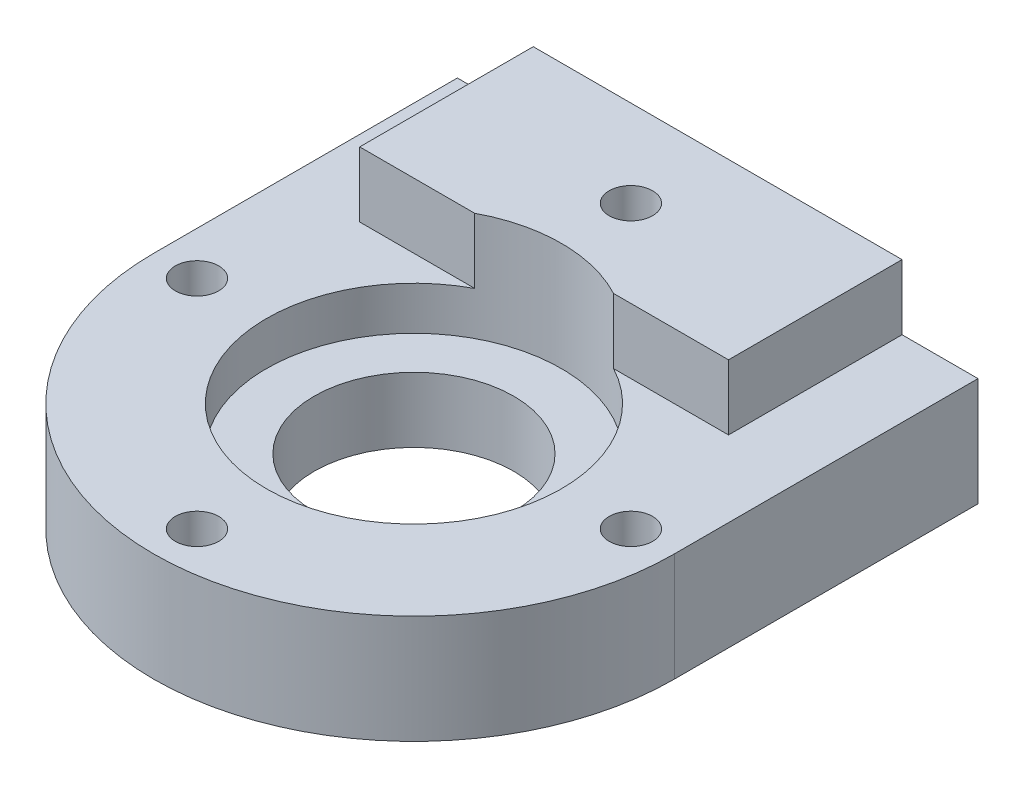
ISO-10303-21;
HEADER;
FILE_DESCRIPTION(('STEP AP214'),'2;1');
FILE_NAME('part.step','',(''),(''),'','','');
FILE_SCHEMA(('AUTOMOTIVE_DESIGN { 1 0 10303 214 1 1 1 1 }'));
ENDSEC;
DATA;
#1=APPLICATION_CONTEXT('core data for automotive mechanical design processes');
#2=APPLICATION_PROTOCOL_DEFINITION('international standard','automotive_design',2000,#1);
#3=PRODUCT_CONTEXT('',#1,'mechanical');
#4=PRODUCT('Part','Part','',(#3));
#5=PRODUCT_RELATED_PRODUCT_CATEGORY('part','',(#4));
#6=PRODUCT_DEFINITION_FORMATION('','',#4);
#7=PRODUCT_DEFINITION_CONTEXT('part definition',#1,'design');
#8=PRODUCT_DEFINITION('design','',#6,#7);
#9=PRODUCT_DEFINITION_SHAPE('','',#8);
#10=(LENGTH_UNIT() NAMED_UNIT(*) SI_UNIT(.MILLI.,.METRE.));
#11=(NAMED_UNIT(*) PLANE_ANGLE_UNIT() SI_UNIT($,.RADIAN.));
#12=(NAMED_UNIT(*) SI_UNIT($,.STERADIAN.) SOLID_ANGLE_UNIT());
#13=UNCERTAINTY_MEASURE_WITH_UNIT(LENGTH_MEASURE(1.E-05),#10,'distance_accuracy_value','');
#14=(GEOMETRIC_REPRESENTATION_CONTEXT(3) GLOBAL_UNCERTAINTY_ASSIGNED_CONTEXT((#13)) GLOBAL_UNIT_ASSIGNED_CONTEXT((#10,
#11,#12)) REPRESENTATION_CONTEXT('',''));
#15=CARTESIAN_POINT('',(0.,0.,0.));
#16=DIRECTION('',(0.,0.,1.));
#17=DIRECTION('',(1.,0.,0.));
#18=AXIS2_PLACEMENT_3D('',#15,#16,#17);
#19=CARTESIAN_POINT('',(0.,0.,5.00000000000002));
#20=DIRECTION('',(0.,0.,1.));
#21=DIRECTION('',(1.,0.,0.));
#22=AXIS2_PLACEMENT_3D('',#19,#20,#21);
#23=PLANE('',#22);
#24=DIRECTION('',(-1.,0.,0.));
#25=VECTOR('',#24,1.);
#26=CARTESIAN_POINT('',(42.5,25.,5.00000000000002));
#27=LINE('',#26,#25);
#28=CARTESIAN_POINT('',(-15.9999999999996,25.,5.00000000000002));
#29=VERTEX_POINT('',#28);
#30=CARTESIAN_POINT('',(-42.5,25.,5.00000000000002));
#31=VERTEX_POINT('',#30);
#32=EDGE_CURVE('E216',#29,#31,#27,.T.);
#33=ORIENTED_EDGE('',*,*,#32,.F.);
#34=DIRECTION('',(0.,-1.,0.));
#35=VECTOR('',#34,1.);
#36=CARTESIAN_POINT('',(-15.9999999999996,65.,5.00000000000002));
#37=LINE('',#36,#35);
#38=CARTESIAN_POINT('',(-15.9999999999996,40.,5.00000000000002));
#39=VERTEX_POINT('',#38);
#40=EDGE_CURVE('E11',#29,#39,#37,.F.);
#41=ORIENTED_EDGE('',*,*,#40,.T.);
#42=DIRECTION('',(1.,0.,0.));
#43=VECTOR('',#42,1.);
#44=CARTESIAN_POINT('',(42.5,40.,5.00000000000002));
#45=LINE('',#44,#43);
#46=CARTESIAN_POINT('',(-42.5,40.,5.00000000000002));
#47=VERTEX_POINT('',#46);
#48=EDGE_CURVE('E126',#47,#39,#45,.T.);
#49=ORIENTED_EDGE('',*,*,#48,.F.);
#50=DIRECTION('',(0.,1.,0.));
#51=VECTOR('',#50,1.);
#52=CARTESIAN_POINT('',(-42.5,25.,5.00000000000002));
#53=LINE('',#52,#51);
#54=EDGE_CURVE('E131',#31,#47,#53,.T.);
#55=ORIENTED_EDGE('',*,*,#54,.F.);
#56=EDGE_LOOP('',(#33,#41,#49,#55));
#57=FACE_BOUND('',#56,.T.);
#58=ADVANCED_FACE('F39',(#57),#23,.T.);
#59=CARTESIAN_POINT('',(15.9999999999996,40.,5.00000000000002));
#60=VERTEX_POINT('',#59);
#61=CARTESIAN_POINT('',(42.5,40.,5.00000000000002));
#62=VERTEX_POINT('',#61);
#63=EDGE_CURVE('E121',#60,#62,#45,.T.);
#64=ORIENTED_EDGE('',*,*,#63,.F.);
#65=DIRECTION('',(0.,-1.,0.));
#66=VECTOR('',#65,1.);
#67=CARTESIAN_POINT('',(15.9999999999996,65.,5.00000000000002));
#68=LINE('',#67,#66);
#69=CARTESIAN_POINT('',(15.9999999999996,25.,5.00000000000002));
#70=VERTEX_POINT('',#69);
#71=EDGE_CURVE('E50',#60,#70,#68,.T.);
#72=ORIENTED_EDGE('',*,*,#71,.T.);
#73=CARTESIAN_POINT('',(42.5,25.,5.00000000000002));
#74=VERTEX_POINT('',#73);
#75=EDGE_CURVE('E139',#74,#70,#27,.T.);
#76=ORIENTED_EDGE('',*,*,#75,.F.);
#77=DIRECTION('',(0.,-1.,0.));
#78=VECTOR('',#77,1.);
#79=CARTESIAN_POINT('',(42.5,25.,5.00000000000002));
#80=LINE('',#79,#78);
#81=EDGE_CURVE('E135',#62,#74,#80,.T.);
#82=ORIENTED_EDGE('',*,*,#81,.F.);
#83=EDGE_LOOP('',(#64,#72,#76,#82));
#84=FACE_BOUND('',#83,.T.);
#85=ADVANCED_FACE('F134',(#84),#23,.T.);
#86=CARTESIAN_POINT('',(0.,25.,35.));
#87=DIRECTION('',(0.,-1.,0.));
#88=DIRECTION('',(0.,0.,-1.));
#89=AXIS2_PLACEMENT_3D('',#86,#87,#88);
#90=CYLINDRICAL_SURFACE('',#89,60.);
#91=CARTESIAN_POINT('',(0.,0.,35.));
#92=DIRECTION('',(0.,1.,0.));
#93=DIRECTION('',(0.,0.,1.));
#94=AXIS2_PLACEMENT_3D('',#91,#92,#93);
#95=CIRCLE('',#94,60.);
#96=CARTESIAN_POINT('',(-60.,0.,35.));
#97=VERTEX_POINT('',#96);
#98=CARTESIAN_POINT('',(60.,0.,35.));
#99=VERTEX_POINT('',#98);
#100=EDGE_CURVE('E153',#97,#99,#95,.T.);
#101=ORIENTED_EDGE('',*,*,#100,.T.);
#102=DIRECTION('',(0.,-1.,0.));
#103=VECTOR('',#102,1.);
#104=CARTESIAN_POINT('',(60.,25.,35.));
#105=LINE('',#104,#103);
#106=CARTESIAN_POINT('',(60.,25.,35.));
#107=VERTEX_POINT('',#106);
#108=EDGE_CURVE('E122',#107,#99,#105,.T.);
#109=ORIENTED_EDGE('',*,*,#108,.F.);
#110=CARTESIAN_POINT('',(0.,25.,35.));
#111=DIRECTION('',(0.,1.,0.));
#112=DIRECTION('',(0.,0.,1.));
#113=AXIS2_PLACEMENT_3D('',#110,#111,#112);
#114=CIRCLE('',#113,60.);
#115=CARTESIAN_POINT('',(-60.,25.,35.));
#116=VERTEX_POINT('',#115);
#117=EDGE_CURVE('E157',#116,#107,#114,.T.);
#118=ORIENTED_EDGE('',*,*,#117,.F.);
#119=DIRECTION('',(0.,-1.,0.));
#120=VECTOR('',#119,1.);
#121=CARTESIAN_POINT('',(-60.,25.,35.));
#122=LINE('',#121,#120);
#123=EDGE_CURVE('E173',#116,#97,#122,.T.);
#124=ORIENTED_EDGE('',*,*,#123,.T.);
#125=EDGE_LOOP('',(#101,#109,#118,#124));
#126=FACE_BOUND('',#125,.T.);
#127=ADVANCED_FACE('F41',(#126),#90,.T.);
#128=CARTESIAN_POINT('',(60.,25.,-35.));
#129=DIRECTION('',(-1.,0.,0.));
#130=DIRECTION('',(0.,0.,1.));
#131=AXIS2_PLACEMENT_3D('',#128,#129,#130);
#132=PLANE('',#131);
#133=DIRECTION('',(0.,0.,-1.));
#134=VECTOR('',#133,1.);
#135=CARTESIAN_POINT('',(60.,0.,-35.));
#136=LINE('',#135,#134);
#137=CARTESIAN_POINT('',(60.,0.,-35.));
#138=VERTEX_POINT('',#137);
#139=EDGE_CURVE('E175',#99,#138,#136,.T.);
#140=ORIENTED_EDGE('',*,*,#139,.T.);
#141=DIRECTION('',(0.,-1.,0.));
#142=VECTOR('',#141,1.);
#143=CARTESIAN_POINT('',(60.,25.,-35.));
#144=LINE('',#143,#142);
#145=CARTESIAN_POINT('',(60.,25.,-35.));
#146=VERTEX_POINT('',#145);
#147=EDGE_CURVE('E184',#146,#138,#144,.T.);
#148=ORIENTED_EDGE('',*,*,#147,.F.);
#149=DIRECTION('',(0.,0.,-1.));
#150=VECTOR('',#149,1.);
#151=CARTESIAN_POINT('',(60.,25.,-35.));
#152=LINE('',#151,#150);
#153=EDGE_CURVE('E165',#107,#146,#152,.T.);
#154=ORIENTED_EDGE('',*,*,#153,.F.);
#155=ORIENTED_EDGE('',*,*,#108,.T.);
#156=EDGE_LOOP('',(#140,#148,#154,#155));
#157=FACE_BOUND('',#156,.T.);
#158=ADVANCED_FACE('F186',(#157),#132,.F.);
#159=CARTESIAN_POINT('',(-60.,25.,-35.));
#160=DIRECTION('',(0.,0.,1.));
#161=DIRECTION('',(1.,0.,0.));
#162=AXIS2_PLACEMENT_3D('',#159,#160,#161);
#163=PLANE('',#162);
#164=DIRECTION('',(-1.,0.,0.));
#165=VECTOR('',#164,1.);
#166=CARTESIAN_POINT('',(-60.,0.,-35.));
#167=LINE('',#166,#165);
#168=CARTESIAN_POINT('',(-60.,0.,-35.));
#169=VERTEX_POINT('',#168);
#170=EDGE_CURVE('E177',#138,#169,#167,.T.);
#171=ORIENTED_EDGE('',*,*,#170,.T.);
#172=DIRECTION('',(0.,-1.,0.));
#173=VECTOR('',#172,1.);
#174=CARTESIAN_POINT('',(-60.,25.,-35.));
#175=LINE('',#174,#173);
#176=CARTESIAN_POINT('',(-60.,25.,-35.));
#177=VERTEX_POINT('',#176);
#178=EDGE_CURVE('E182',#177,#169,#175,.T.);
#179=ORIENTED_EDGE('',*,*,#178,.F.);
#180=DIRECTION('',(-1.,0.,0.));
#181=VECTOR('',#180,1.);
#182=CARTESIAN_POINT('',(-60.,25.,-35.));
#183=LINE('',#182,#181);
#184=CARTESIAN_POINT('',(-42.5,25.,-35.));
#185=VERTEX_POINT('',#184);
#186=EDGE_CURVE('E164',#185,#177,#183,.T.);
#187=ORIENTED_EDGE('',*,*,#186,.F.);
#188=DIRECTION('',(0.,1.,0.));
#189=VECTOR('',#188,1.);
#190=CARTESIAN_POINT('',(-42.5,25.,-35.));
#191=LINE('',#190,#189);
#192=CARTESIAN_POINT('',(-42.5,40.,-35.));
#193=VERTEX_POINT('',#192);
#194=EDGE_CURVE('E64',#185,#193,#191,.T.);
#195=ORIENTED_EDGE('',*,*,#194,.T.);
#196=DIRECTION('',(1.,0.,0.));
#197=VECTOR('',#196,1.);
#198=CARTESIAN_POINT('',(42.5,40.,-35.));
#199=LINE('',#198,#197);
#200=CARTESIAN_POINT('',(42.5,40.,-35.));
#201=VERTEX_POINT('',#200);
#202=EDGE_CURVE('E146',#193,#201,#199,.T.);
#203=ORIENTED_EDGE('',*,*,#202,.T.);
#204=DIRECTION('',(0.,-1.,0.));
#205=VECTOR('',#204,1.);
#206=CARTESIAN_POINT('',(42.5,25.,-35.));
#207=LINE('',#206,#205);
#208=CARTESIAN_POINT('',(42.5,25.,-35.));
#209=VERTEX_POINT('',#208);
#210=EDGE_CURVE('E141',#201,#209,#207,.T.);
#211=ORIENTED_EDGE('',*,*,#210,.T.);
#212=EDGE_CURVE('E167',#146,#209,#183,.T.);
#213=ORIENTED_EDGE('',*,*,#212,.F.);
#214=ORIENTED_EDGE('',*,*,#147,.T.);
#215=EDGE_LOOP('',(#171,#179,#187,#195,#203,#211,#213,#214));
#216=FACE_BOUND('',#215,.T.);
#217=ADVANCED_FACE('F205',(#216),#163,.F.);
#218=CARTESIAN_POINT('',(-60.,25.,-35.));
#219=DIRECTION('',(1.,0.,0.));
#220=DIRECTION('',(0.,0.,-1.));
#221=AXIS2_PLACEMENT_3D('',#218,#219,#220);
#222=PLANE('',#221);
#223=DIRECTION('',(0.,0.,1.));
#224=VECTOR('',#223,1.);
#225=CARTESIAN_POINT('',(-60.,0.,-35.));
#226=LINE('',#225,#224);
#227=EDGE_CURVE('E162',#169,#97,#226,.T.);
#228=ORIENTED_EDGE('',*,*,#227,.T.);
#229=ORIENTED_EDGE('',*,*,#123,.F.);
#230=DIRECTION('',(0.,0.,1.));
#231=VECTOR('',#230,1.);
#232=CARTESIAN_POINT('',(-60.,25.,-35.));
#233=LINE('',#232,#231);
#234=EDGE_CURVE('E166',#177,#116,#233,.T.);
#235=ORIENTED_EDGE('',*,*,#234,.F.);
#236=ORIENTED_EDGE('',*,*,#178,.T.);
#237=EDGE_LOOP('',(#228,#229,#235,#236));
#238=FACE_BOUND('',#237,.T.);
#239=ADVANCED_FACE('F210',(#238),#222,.F.);
#240=CARTESIAN_POINT('',(0.,25.,35.));
#241=DIRECTION('',(0.,1.,0.));
#242=DIRECTION('',(0.,0.,1.));
#243=AXIS2_PLACEMENT_3D('',#240,#241,#242);
#244=PLANE('',#243);
#245=CARTESIAN_POINT('',(-50.,25.,35.0000000000002));
#246=DIRECTION('',(0.,1.,0.));
#247=DIRECTION('',(0.,0.,1.));
#248=AXIS2_PLACEMENT_3D('',#245,#246,#247);
#249=CIRCLE('',#248,5.);
#250=CARTESIAN_POINT('',(-50.,25.,40.0000000000002));
#251=VERTEX_POINT('',#250);
#252=EDGE_CURVE('E148',#251,#251,#249,.T.);
#253=ORIENTED_EDGE('',*,*,#252,.F.);
#254=EDGE_LOOP('',(#253));
#255=FACE_BOUND('',#254,.T.);
#256=CARTESIAN_POINT('',(50.,25.,35.0000000000002));
#257=DIRECTION('',(0.,1.,0.));
#258=DIRECTION('',(0.,0.,1.));
#259=AXIS2_PLACEMENT_3D('',#256,#257,#258);
#260=CIRCLE('',#259,5.);
#261=CARTESIAN_POINT('',(50.,25.,40.0000000000002));
#262=VERTEX_POINT('',#261);
#263=EDGE_CURVE('E222',#262,#262,#260,.T.);
#264=ORIENTED_EDGE('',*,*,#263,.F.);
#265=EDGE_LOOP('',(#264));
#266=FACE_BOUND('',#265,.T.);
#267=CARTESIAN_POINT('',(0.,25.,85.0000000000002));
#268=DIRECTION('',(0.,1.,0.));
#269=DIRECTION('',(0.,0.,1.));
#270=AXIS2_PLACEMENT_3D('',#267,#268,#269);
#271=CIRCLE('',#270,5.);
#272=CARTESIAN_POINT('',(0.,25.,90.0000000000002));
#273=VERTEX_POINT('',#272);
#274=EDGE_CURVE('E221',#273,#273,#271,.T.);
#275=ORIENTED_EDGE('',*,*,#274,.F.);
#276=EDGE_LOOP('',(#275));
#277=FACE_BOUND('',#276,.T.);
#278=ORIENTED_EDGE('',*,*,#75,.T.);
#279=CARTESIAN_POINT('',(0.,25.,35.0000000000002));
#280=DIRECTION('',(0.,1.,0.));
#281=DIRECTION('',(0.,0.,1.));
#282=AXIS2_PLACEMENT_3D('',#279,#280,#281);
#283=CIRCLE('',#282,34.);
#284=EDGE_CURVE('E53',#70,#29,#283,.F.);
#285=ORIENTED_EDGE('',*,*,#284,.T.);
#286=ORIENTED_EDGE('',*,*,#32,.T.);
#287=DIRECTION('',(0.,0.,-1.));
#288=VECTOR('',#287,1.);
#289=CARTESIAN_POINT('',(-42.5,25.,5.00000000000002));
#290=LINE('',#289,#288);
#291=EDGE_CURVE('E156',#31,#185,#290,.T.);
#292=ORIENTED_EDGE('',*,*,#291,.T.);
#293=ORIENTED_EDGE('',*,*,#186,.T.);
#294=ORIENTED_EDGE('',*,*,#234,.T.);
#295=ORIENTED_EDGE('',*,*,#117,.T.);
#296=ORIENTED_EDGE('',*,*,#153,.T.);
#297=ORIENTED_EDGE('',*,*,#212,.T.);
#298=DIRECTION('',(0.,0.,-1.));
#299=VECTOR('',#298,1.);
#300=CARTESIAN_POINT('',(42.5,25.,5.00000000000002));
#301=LINE('',#300,#299);
#302=EDGE_CURVE('E140',#74,#209,#301,.T.);
#303=ORIENTED_EDGE('',*,*,#302,.F.);
#304=EDGE_LOOP('',(#278,#285,#286,#292,#293,#294,#295,#296,#297,#303));
#305=FACE_BOUND('',#304,.T.);
#306=ADVANCED_FACE('F207',(#255,#266,#277,#305),#244,.T.);
#307=CARTESIAN_POINT('',(0.,0.,35.));
#308=DIRECTION('',(0.,1.,0.));
#309=DIRECTION('',(0.,0.,1.));
#310=AXIS2_PLACEMENT_3D('',#307,#308,#309);
#311=PLANE('',#310);
#312=CARTESIAN_POINT('',(0.,0.,35.0000000000002));
#313=DIRECTION('',(0.,1.,0.));
#314=DIRECTION('',(0.,0.,1.));
#315=AXIS2_PLACEMENT_3D('',#312,#313,#314);
#316=CIRCLE('',#315,23.);
#317=CARTESIAN_POINT('',(0.,0.,58.0000000000002));
#318=VERTEX_POINT('',#317);
#319=EDGE_CURVE('E241',#318,#318,#316,.T.);
#320=ORIENTED_EDGE('',*,*,#319,.T.);
#321=EDGE_LOOP('',(#320));
#322=FACE_BOUND('',#321,.T.);
#323=CARTESIAN_POINT('',(0.,0.,-15.));
#324=DIRECTION('',(0.,1.,0.));
#325=DIRECTION('',(0.,0.,1.));
#326=AXIS2_PLACEMENT_3D('',#323,#324,#325);
#327=CIRCLE('',#326,5.);
#328=CARTESIAN_POINT('',(0.,0.,-9.99999999999998));
#329=VERTEX_POINT('',#328);
#330=EDGE_CURVE('E229',#329,#329,#327,.T.);
#331=ORIENTED_EDGE('',*,*,#330,.T.);
#332=EDGE_LOOP('',(#331));
#333=FACE_BOUND('',#332,.T.);
#334=CARTESIAN_POINT('',(-50.,0.,35.0000000000002));
#335=DIRECTION('',(0.,1.,0.));
#336=DIRECTION('',(0.,0.,1.));
#337=AXIS2_PLACEMENT_3D('',#334,#335,#336);
#338=CIRCLE('',#337,5.);
#339=CARTESIAN_POINT('',(-50.,0.,40.0000000000002));
#340=VERTEX_POINT('',#339);
#341=EDGE_CURVE('E234',#340,#340,#338,.T.);
#342=ORIENTED_EDGE('',*,*,#341,.T.);
#343=EDGE_LOOP('',(#342));
#344=FACE_BOUND('',#343,.T.);
#345=CARTESIAN_POINT('',(50.,0.,35.0000000000002));
#346=DIRECTION('',(0.,1.,0.));
#347=DIRECTION('',(0.,0.,1.));
#348=AXIS2_PLACEMENT_3D('',#345,#346,#347);
#349=CIRCLE('',#348,5.);
#350=CARTESIAN_POINT('',(50.,0.,40.0000000000002));
#351=VERTEX_POINT('',#350);
#352=EDGE_CURVE('E232',#351,#351,#349,.T.);
#353=ORIENTED_EDGE('',*,*,#352,.T.);
#354=EDGE_LOOP('',(#353));
#355=FACE_BOUND('',#354,.T.);
#356=CARTESIAN_POINT('',(0.,0.,85.0000000000002));
#357=DIRECTION('',(0.,1.,0.));
#358=DIRECTION('',(0.,0.,1.));
#359=AXIS2_PLACEMENT_3D('',#356,#357,#358);
#360=CIRCLE('',#359,5.);
#361=CARTESIAN_POINT('',(0.,0.,90.0000000000002));
#362=VERTEX_POINT('',#361);
#363=EDGE_CURVE('E227',#362,#362,#360,.T.);
#364=ORIENTED_EDGE('',*,*,#363,.T.);
#365=EDGE_LOOP('',(#364));
#366=FACE_BOUND('',#365,.T.);
#367=ORIENTED_EDGE('',*,*,#100,.F.);
#368=ORIENTED_EDGE('',*,*,#227,.F.);
#369=ORIENTED_EDGE('',*,*,#170,.F.);
#370=ORIENTED_EDGE('',*,*,#139,.F.);
#371=EDGE_LOOP('',(#367,#368,#369,#370));
#372=FACE_BOUND('',#371,.T.);
#373=ADVANCED_FACE('F196',(#322,#333,#344,#355,#366,#372),#311,.F.);
#374=CARTESIAN_POINT('',(42.5,25.,5.00000000000002));
#375=DIRECTION('',(1.,0.,0.));
#376=DIRECTION('',(0.,0.,-1.));
#377=AXIS2_PLACEMENT_3D('',#374,#375,#376);
#378=PLANE('',#377);
#379=ORIENTED_EDGE('',*,*,#210,.F.);
#380=DIRECTION('',(0.,0.,-1.));
#381=VECTOR('',#380,1.);
#382=CARTESIAN_POINT('',(42.5,40.,5.00000000000002));
#383=LINE('',#382,#381);
#384=EDGE_CURVE('E151',#62,#201,#383,.T.);
#385=ORIENTED_EDGE('',*,*,#384,.F.);
#386=ORIENTED_EDGE('',*,*,#81,.T.);
#387=ORIENTED_EDGE('',*,*,#302,.T.);
#388=EDGE_LOOP('',(#379,#385,#386,#387));
#389=FACE_BOUND('',#388,.T.);
#390=ADVANCED_FACE('F213',(#389),#378,.T.);
#391=CARTESIAN_POINT('',(42.5,40.,5.00000000000002));
#392=DIRECTION('',(0.,1.,0.));
#393=DIRECTION('',(0.,0.,1.));
#394=AXIS2_PLACEMENT_3D('',#391,#392,#393);
#395=PLANE('',#394);
#396=CARTESIAN_POINT('',(0.,40.,-15.));
#397=DIRECTION('',(0.,1.,0.));
#398=DIRECTION('',(0.,0.,1.));
#399=AXIS2_PLACEMENT_3D('',#396,#397,#398);
#400=CIRCLE('',#399,5.);
#401=CARTESIAN_POINT('',(0.,40.,-9.99999999999998));
#402=VERTEX_POINT('',#401);
#403=EDGE_CURVE('E240',#402,#402,#400,.T.);
#404=ORIENTED_EDGE('',*,*,#403,.F.);
#405=EDGE_LOOP('',(#404));
#406=FACE_BOUND('',#405,.T.);
#407=ORIENTED_EDGE('',*,*,#48,.T.);
#408=CARTESIAN_POINT('',(0.,40.,35.0000000000002));
#409=DIRECTION('',(0.,1.,0.));
#410=DIRECTION('',(0.,0.,1.));
#411=AXIS2_PLACEMENT_3D('',#408,#409,#410);
#412=CIRCLE('',#411,34.);
#413=EDGE_CURVE('E119',#39,#60,#412,.F.);
#414=ORIENTED_EDGE('',*,*,#413,.T.);
#415=ORIENTED_EDGE('',*,*,#63,.T.);
#416=ORIENTED_EDGE('',*,*,#384,.T.);
#417=ORIENTED_EDGE('',*,*,#202,.F.);
#418=DIRECTION('',(0.,0.,-1.));
#419=VECTOR('',#418,1.);
#420=CARTESIAN_POINT('',(-42.5,40.,5.00000000000002));
#421=LINE('',#420,#419);
#422=EDGE_CURVE('E152',#47,#193,#421,.T.);
#423=ORIENTED_EDGE('',*,*,#422,.F.);
#424=EDGE_LOOP('',(#407,#414,#415,#416,#417,#423));
#425=FACE_BOUND('',#424,.T.);
#426=ADVANCED_FACE('F124',(#406,#425),#395,.T.);
#427=CARTESIAN_POINT('',(-42.5,25.,5.00000000000002));
#428=DIRECTION('',(-1.,0.,0.));
#429=DIRECTION('',(0.,0.,1.));
#430=AXIS2_PLACEMENT_3D('',#427,#428,#429);
#431=PLANE('',#430);
#432=ORIENTED_EDGE('',*,*,#194,.F.);
#433=ORIENTED_EDGE('',*,*,#291,.F.);
#434=ORIENTED_EDGE('',*,*,#54,.T.);
#435=ORIENTED_EDGE('',*,*,#422,.T.);
#436=EDGE_LOOP('',(#432,#433,#434,#435));
#437=FACE_BOUND('',#436,.T.);
#438=ADVANCED_FACE('F288',(#437),#431,.T.);
#439=CARTESIAN_POINT('',(0.,0.,-15.));
#440=DIRECTION('',(0.,1.,0.));
#441=DIRECTION('',(0.,0.,1.));
#442=AXIS2_PLACEMENT_3D('',#439,#440,#441);
#443=CYLINDRICAL_SURFACE('',#442,5.);
#444=ORIENTED_EDGE('',*,*,#330,.F.);
#445=EDGE_LOOP('',(#444));
#446=FACE_BOUND('',#445,.T.);
#447=ORIENTED_EDGE('',*,*,#403,.T.);
#448=EDGE_LOOP('',(#447));
#449=FACE_BOUND('',#448,.T.);
#450=ADVANCED_FACE('F295',(#446,#449),#443,.F.);
#451=CARTESIAN_POINT('',(0.,0.,85.0000000000002));
#452=DIRECTION('',(0.,1.,0.));
#453=DIRECTION('',(0.,0.,1.));
#454=AXIS2_PLACEMENT_3D('',#451,#452,#453);
#455=CYLINDRICAL_SURFACE('',#454,5.);
#456=ORIENTED_EDGE('',*,*,#274,.T.);
#457=EDGE_LOOP('',(#456));
#458=FACE_BOUND('',#457,.T.);
#459=ORIENTED_EDGE('',*,*,#363,.F.);
#460=EDGE_LOOP('',(#459));
#461=FACE_BOUND('',#460,.T.);
#462=ADVANCED_FACE('F281',(#458,#461),#455,.F.);
#463=CARTESIAN_POINT('',(50.,0.,35.0000000000002));
#464=DIRECTION('',(0.,1.,0.));
#465=DIRECTION('',(0.,0.,1.));
#466=AXIS2_PLACEMENT_3D('',#463,#464,#465);
#467=CYLINDRICAL_SURFACE('',#466,5.);
#468=ORIENTED_EDGE('',*,*,#263,.T.);
#469=EDGE_LOOP('',(#468));
#470=FACE_BOUND('',#469,.T.);
#471=ORIENTED_EDGE('',*,*,#352,.F.);
#472=EDGE_LOOP('',(#471));
#473=FACE_BOUND('',#472,.T.);
#474=ADVANCED_FACE('F272',(#470,#473),#467,.F.);
#475=CARTESIAN_POINT('',(-50.,0.,35.0000000000002));
#476=DIRECTION('',(0.,1.,0.));
#477=DIRECTION('',(0.,0.,1.));
#478=AXIS2_PLACEMENT_3D('',#475,#476,#477);
#479=CYLINDRICAL_SURFACE('',#478,5.);
#480=ORIENTED_EDGE('',*,*,#252,.T.);
#481=EDGE_LOOP('',(#480));
#482=FACE_BOUND('',#481,.T.);
#483=ORIENTED_EDGE('',*,*,#341,.F.);
#484=EDGE_LOOP('',(#483));
#485=FACE_BOUND('',#484,.T.);
#486=ADVANCED_FACE('F266',(#482,#485),#479,.F.);
#487=CARTESIAN_POINT('',(0.,65.,35.0000000000002));
#488=DIRECTION('',(0.,-1.,0.));
#489=DIRECTION('',(0.,0.,-1.));
#490=AXIS2_PLACEMENT_3D('',#487,#488,#489);
#491=CYLINDRICAL_SURFACE('',#490,34.);
#492=ORIENTED_EDGE('',*,*,#284,.F.);
#493=ORIENTED_EDGE('',*,*,#71,.F.);
#494=ORIENTED_EDGE('',*,*,#413,.F.);
#495=ORIENTED_EDGE('',*,*,#40,.F.);
#496=EDGE_LOOP('',(#492,#493,#494,#495));
#497=FACE_BOUND('',#496,.T.);
#498=CARTESIAN_POINT('',(0.,15.,35.0000000000002));
#499=DIRECTION('',(0.,1.,0.));
#500=DIRECTION('',(0.,0.,1.));
#501=AXIS2_PLACEMENT_3D('',#498,#499,#500);
#502=CIRCLE('',#501,34.);
#503=CARTESIAN_POINT('',(0.,15.,69.0000000000002));
#504=VERTEX_POINT('',#503);
#505=EDGE_CURVE('E129',#504,#504,#502,.T.);
#506=ORIENTED_EDGE('',*,*,#505,.F.);
#507=EDGE_LOOP('',(#506));
#508=FACE_BOUND('',#507,.T.);
#509=ADVANCED_FACE('F113',(#497,#508),#491,.F.);
#510=CARTESIAN_POINT('',(0.,15.,35.0000000000002));
#511=DIRECTION('',(0.,1.,0.));
#512=DIRECTION('',(0.,0.,1.));
#513=AXIS2_PLACEMENT_3D('',#510,#511,#512);
#514=PLANE('',#513);
#515=CARTESIAN_POINT('',(0.,15.,35.0000000000002));
#516=DIRECTION('',(0.,1.,0.));
#517=DIRECTION('',(0.,0.,1.));
#518=AXIS2_PLACEMENT_3D('',#515,#516,#517);
#519=CIRCLE('',#518,23.);
#520=CARTESIAN_POINT('',(0.,15.,58.0000000000002));
#521=VERTEX_POINT('',#520);
#522=EDGE_CURVE('E247',#521,#521,#519,.T.);
#523=ORIENTED_EDGE('',*,*,#522,.F.);
#524=EDGE_LOOP('',(#523));
#525=FACE_BOUND('',#524,.T.);
#526=ORIENTED_EDGE('',*,*,#505,.T.);
#527=EDGE_LOOP('',(#526));
#528=FACE_BOUND('',#527,.T.);
#529=ADVANCED_FACE('F260',(#525,#528),#514,.T.);
#530=CARTESIAN_POINT('',(0.,0.,35.0000000000002));
#531=DIRECTION('',(0.,1.,0.));
#532=DIRECTION('',(0.,0.,1.));
#533=AXIS2_PLACEMENT_3D('',#530,#531,#532);
#534=CYLINDRICAL_SURFACE('',#533,23.);
#535=ORIENTED_EDGE('',*,*,#319,.F.);
#536=EDGE_LOOP('',(#535));
#537=FACE_BOUND('',#536,.T.);
#538=ORIENTED_EDGE('',*,*,#522,.T.);
#539=EDGE_LOOP('',(#538));
#540=FACE_BOUND('',#539,.T.);
#541=ADVANCED_FACE('F255',(#537,#540),#534,.F.);
#542=CLOSED_SHELL('',(#58,#85,#127,#158,#217,#239,#306,#373,#390,#426,#438,#450,#462,#474,#486,
#509,#529,#541));
#543=MANIFOLD_SOLID_BREP('B2',#542);
#544=ADVANCED_BREP_SHAPE_REPRESENTATION('',(#18,#543),#14);
#545=SHAPE_DEFINITION_REPRESENTATION(#9,#544);
ENDSEC;
END-ISO-10303-21;
